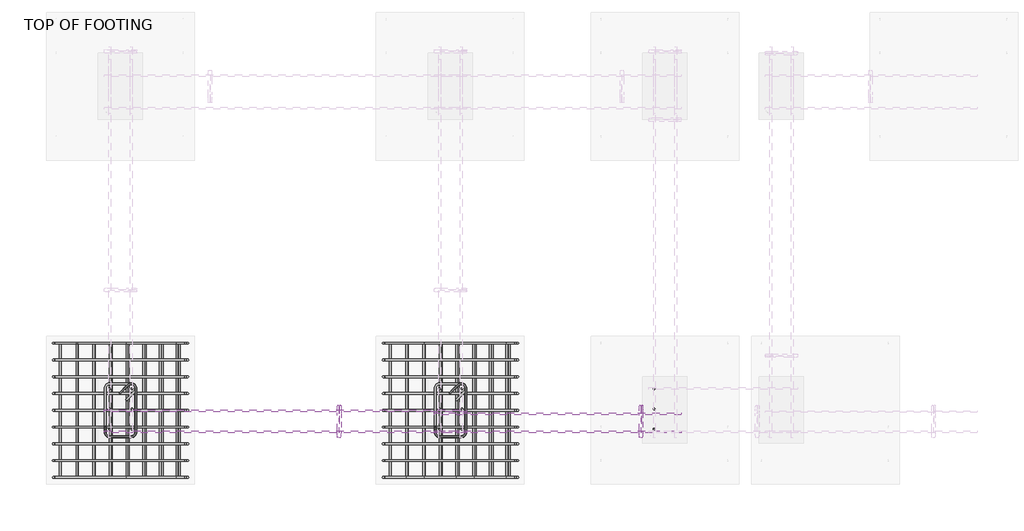
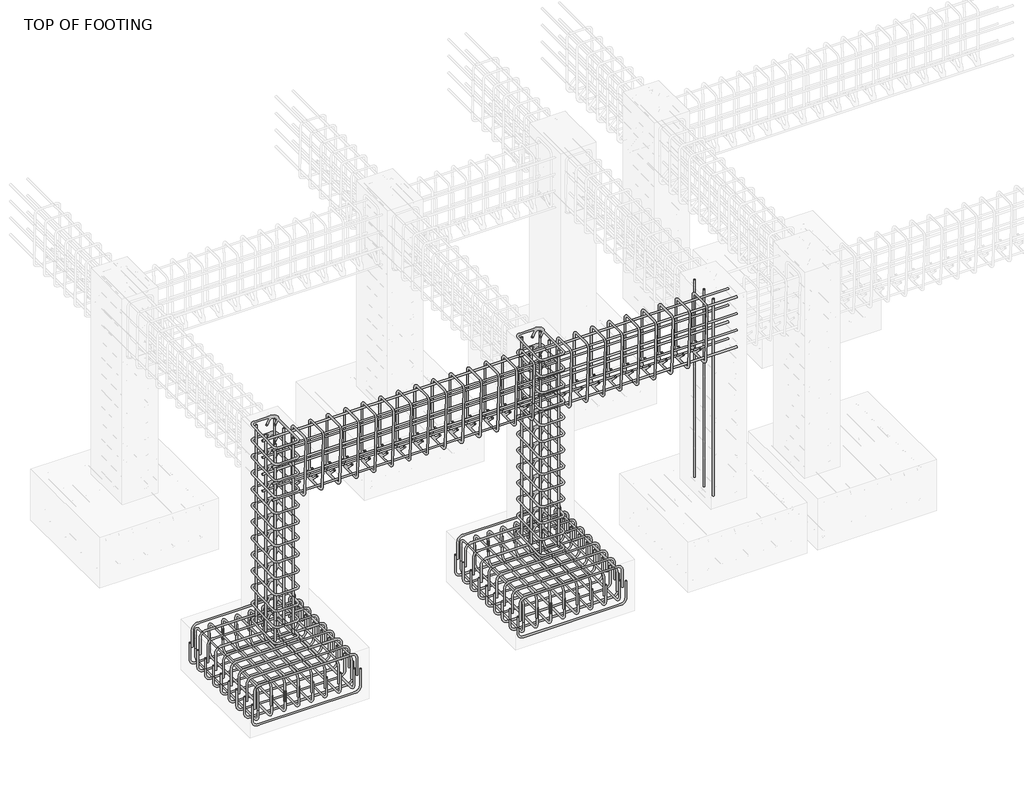
# One storey, part 2 of 19: 21 reinforcing bars.
"""IFC4 building model written with IfcOpenShell, lengths in millimetres."""

from ifc_helpers import new_model, si_unit, point, frame, origin, place, context, project, spatial, polyline, circle_curve, trimmed, segment, composite_curve, source, transform, mapped, element, save
from ifc_brep_helpers import swept_disk

model = new_model("IFC4")

# Units and contexts
model_context = context("Model", 3, world=origin())
ifc_project = project(units=[si_unit("LENGTHUNIT", "METRE", prefix="MILLI")], contexts=[model_context])

# Site, building, storey
site = spatial("IfcSite", under=ifc_project)
building = spatial("IfcBuilding", under=site)
storey = spatial("IfcBuildingStorey", under=building, Name="TOP OF FOOTING", Elevation=-1828.8)

# Reinforcing bars
placement = place(None, origin())
reinforcing_bar_shape = source(origin(), model_context, "Body", "SolidModel", [
    swept_disk(composite_curve([segment(polyline([(-5184.0266954, -464.2751006, -2026.8103972), (-5184.0266954, -464.2751006, -2174.1103972)]), True, "CONTINUOUS"), segment(trimmed(circle_curve(frame((-5230.3766954, -464.2751006, -2174.1103972), z_axis=(0.0, 1.0, 0.0), x_axis=(46.350000000000364, 0.0, 0.0)), 46.35), [point((-5184.0266954, -464.2751006, -2174.1103972))], [point((-5230.3766954, -464.2751006, -2220.4603972))], True, "CARTESIAN"), True, "CONTINUOUS"), segment(polyline([(-5230.3766954, -464.2751006, -2220.4603972), (-6044.9766954, -464.2751006, -2220.4603972)]), True, "CONTINUOUS"), segment(trimmed(circle_curve(frame((-6044.9766954, -464.2751006, -2174.1103972), z_axis=(0.0, 1.0, 0.0), x_axis=(0.0, 0.0, -46.34999999999991)), 46.35), [point((-6044.9766954, -464.2751006, -2220.4603972))], [point((-6091.3266954, -464.2751006, -2174.1103972))], True, "CARTESIAN"), True, "CONTINUOUS"), segment(polyline([(-6091.3266954, -464.2751006, -2174.1103972), (-6091.3266954, -464.2751006, -2026.8103972)]), True, "CONTINUOUS")], self_intersect=False), 6.35),
])
element("IfcReinforcingBar", 1, at=placement, inside=storey, context=model_context, shape_type="MappedRepresentation", body=[
    mapped(reinforcing_bar_shape, transform((0.0, 0.0, 0.0), x_axis=(1.0, 0.0, 0.0), y_axis=(0.0, 1.0, 0.0), z_axis=(0.0, 0.0, 1.0))),
    mapped(reinforcing_bar_shape, transform((0.0, -113.4125, 0.0), x_axis=(1.0, 0.0, 0.0), y_axis=(0.0, 1.0, 0.0), z_axis=(0.0, 0.0, 1.0))),
    mapped(reinforcing_bar_shape, transform((0.0, -226.825, 0.0), x_axis=(1.0, 0.0, 0.0), y_axis=(0.0, 1.0, 0.0), z_axis=(0.0, 0.0, 1.0))),
    mapped(reinforcing_bar_shape, transform((0.0, -340.2375, 0.0), x_axis=(1.0, 0.0, 0.0), y_axis=(0.0, 1.0, 0.0), z_axis=(0.0, 0.0, 1.0))),
    mapped(reinforcing_bar_shape, transform((0.0, -453.65, 0.0), x_axis=(1.0, 0.0, 0.0), y_axis=(0.0, 1.0, 0.0), z_axis=(0.0, 0.0, 1.0))),
    mapped(reinforcing_bar_shape, transform((0.0, -567.0625, 0.0), x_axis=(1.0, 0.0, 0.0), y_axis=(0.0, 1.0, 0.0), z_axis=(0.0, 0.0, 1.0))),
    mapped(reinforcing_bar_shape, transform((0.0, -680.475, 0.0), x_axis=(1.0, 0.0, 0.0), y_axis=(0.0, 1.0, 0.0), z_axis=(0.0, 0.0, 1.0))),
    mapped(reinforcing_bar_shape, transform((0.0, -793.8875, 0.0), x_axis=(1.0, 0.0, 0.0), y_axis=(0.0, 1.0, 0.0), z_axis=(0.0, 0.0, 1.0))),
    mapped(reinforcing_bar_shape, transform((0.0, -907.3, 0.0), x_axis=(1.0, 0.0, 0.0), y_axis=(0.0, 1.0, 0.0), z_axis=(0.0, 0.0, 1.0))),
])
reinforcing_bar_2_shape = source(origin(), model_context, "Body", "SolidModel", [
    swept_disk(composite_curve([segment(polyline([(-6071.7887242, -464.2751006, -2068.8), (-6071.7887242, -464.2751006, -1921.5)]), True, "CONTINUOUS"), segment(trimmed(circle_curve(frame((-6025.4387242, -464.2751006, -1921.5), z_axis=(0.0, 1.0, 0.0), x_axis=(-46.349999999999454, 0.0, 0.0)), 46.35), [point((-6071.7887242, -464.2751006, -1921.5))], [point((-6025.4387242, -464.2751006, -1875.15))], True, "CARTESIAN"), True, "CONTINUOUS"), segment(polyline([(-6025.4387242, -464.2751006, -1875.15), (-5260.3062054, -464.2751006, -1875.15)]), True, "CONTINUOUS"), segment(trimmed(circle_curve(frame((-5260.3062054, -464.2751006, -1921.5), z_axis=(0.0, 1.0, 0.0), x_axis=(0.0, 0.0, 46.34999999999991)), 46.35), [point((-5260.3062054, -464.2751006, -1875.15))], [point((-5213.9562054, -464.2751006, -1921.5))], True, "CARTESIAN"), True, "CONTINUOUS"), segment(polyline([(-5213.9562054, -464.2751006, -1921.5), (-5213.9562054, -464.2751006, -2068.8)]), True, "CONTINUOUS")], self_intersect=False), 6.35),
])
element("IfcReinforcingBar", 2, at=placement, inside=storey, context=model_context, shape_type="MappedRepresentation", body=[
    mapped(reinforcing_bar_2_shape, transform((0.0, 0.0, 0.0), x_axis=(1.0, 0.0, 0.0), y_axis=(0.0, 1.0, 0.0), z_axis=(0.0, 0.0, 1.0))),
    mapped(reinforcing_bar_2_shape, transform((0.0, -113.4125, 0.0), x_axis=(1.0, 0.0, 0.0), y_axis=(0.0, 1.0, 0.0), z_axis=(0.0, 0.0, 1.0))),
    mapped(reinforcing_bar_2_shape, transform((0.0, -226.825, 0.0), x_axis=(1.0, 0.0, 0.0), y_axis=(0.0, 1.0, 0.0), z_axis=(0.0, 0.0, 1.0))),
    mapped(reinforcing_bar_2_shape, transform((0.0, -340.2375, 0.0), x_axis=(1.0, 0.0, 0.0), y_axis=(0.0, 1.0, 0.0), z_axis=(0.0, 0.0, 1.0))),
    mapped(reinforcing_bar_2_shape, transform((0.0, -453.65, 0.0), x_axis=(1.0, 0.0, 0.0), y_axis=(0.0, 1.0, 0.0), z_axis=(0.0, 0.0, 1.0))),
    mapped(reinforcing_bar_2_shape, transform((0.0, -567.0625, 0.0), x_axis=(1.0, 0.0, 0.0), y_axis=(0.0, 1.0, 0.0), z_axis=(0.0, 0.0, 1.0))),
    mapped(reinforcing_bar_2_shape, transform((0.0, -680.475, 0.0), x_axis=(1.0, 0.0, 0.0), y_axis=(0.0, 1.0, 0.0), z_axis=(0.0, 0.0, 1.0))),
    mapped(reinforcing_bar_2_shape, transform((0.0, -793.8875, 0.0), x_axis=(1.0, 0.0, 0.0), y_axis=(0.0, 1.0, 0.0), z_axis=(0.0, 0.0, 1.0))),
    mapped(reinforcing_bar_2_shape, transform((0.0, -907.3, 0.0), x_axis=(1.0, 0.0, 0.0), y_axis=(0.0, 1.0, 0.0), z_axis=(0.0, 0.0, 1.0))),
])
reinforcing_bar_3_shape = source(origin(), model_context, "Body", "SolidModel", [
    swept_disk(composite_curve([segment(polyline([(-5256.531502, -464.2751006, -2090.0818702), (-5256.531502, -464.2751006, -1942.7818702)]), True, "CONTINUOUS"), segment(trimmed(circle_curve(frame((-5256.531502, -510.6251006, -1942.7818702), z_axis=(1.0, 0.0, 0.0), x_axis=(0.0, 46.35000000000002, 0.0)), 46.35), [point((-5256.531502, -464.2751006, -1942.7818702))], [point((-5256.531502, -510.6251006, -1896.4318702))], True, "CARTESIAN"), True, "CONTINUOUS"), segment(polyline([(-5256.531502, -510.6251006, -1896.4318702), (-5256.531502, -1325.2251006, -1896.4318702)]), True, "CONTINUOUS"), segment(trimmed(circle_curve(frame((-5256.531502, -1325.2251006, -1942.7818702), z_axis=(1.0, 0.0, 0.0), x_axis=(0.0, 0.0, 46.34999999999991)), 46.35), [point((-5256.531502, -1325.2251006, -1896.4318702))], [point((-5256.531502, -1371.5751006, -1942.7818702))], True, "CARTESIAN"), True, "CONTINUOUS"), segment(polyline([(-5256.531502, -1371.5751006, -1942.7818702), (-5256.531502, -1371.5751006, -2090.0818702)]), True, "CONTINUOUS")], self_intersect=False), 6.35),
])
element("IfcReinforcingBar", 3, at=placement, inside=storey, context=model_context, shape_type="MappedRepresentation", body=[
    mapped(reinforcing_bar_3_shape, transform((0.0, 0.0, 0.0), x_axis=(1.0, 0.0, 0.0), y_axis=(0.0, 1.0, 0.0), z_axis=(0.0, 0.0, 1.0))),
    mapped(reinforcing_bar_3_shape, transform((-112.5756498, 0.0, 0.0), x_axis=(1.0, 0.0, 0.0), y_axis=(0.0, 1.0, 0.0), z_axis=(0.0, 0.0, 1.0))),
    mapped(reinforcing_bar_3_shape, transform((-225.1512997, 0.0, 0.0), x_axis=(1.0, 0.0, 0.0), y_axis=(0.0, 1.0, 0.0), z_axis=(0.0, 0.0, 1.0))),
    mapped(reinforcing_bar_3_shape, transform((-337.7269495, 0.0, 0.0), x_axis=(1.0, 0.0, 0.0), y_axis=(0.0, 1.0, 0.0), z_axis=(0.0, 0.0, 1.0))),
    mapped(reinforcing_bar_3_shape, transform((-450.3025994, 0.0, 0.0), x_axis=(1.0, 0.0, 0.0), y_axis=(0.0, 1.0, 0.0), z_axis=(0.0, 0.0, 1.0))),
    mapped(reinforcing_bar_3_shape, transform((-562.8782492, 0.0, 0.0), x_axis=(1.0, 0.0, 0.0), y_axis=(0.0, 1.0, 0.0), z_axis=(0.0, 0.0, 1.0))),
    mapped(reinforcing_bar_3_shape, transform((-675.4538991, 0.0, 0.0), x_axis=(1.0, 0.0, 0.0), y_axis=(0.0, 1.0, 0.0), z_axis=(0.0, 0.0, 1.0))),
    mapped(reinforcing_bar_3_shape, transform((-788.0295489, 0.0, 0.0), x_axis=(1.0, 0.0, 0.0), y_axis=(0.0, 1.0, 0.0), z_axis=(0.0, 0.0, 1.0))),
])
reinforcing_bar_4_shape = source(origin(), model_context, "Body", "SolidModel", [
    swept_disk(composite_curve([segment(polyline([(-6044.5610509, -464.2751006, -2000.9061905), (-6044.5610509, -464.2751006, -2148.2061905)]), True, "CONTINUOUS"), segment(trimmed(circle_curve(frame((-6044.5610509, -510.6251006, -2148.2061905), z_axis=(-1.0, 0.0, 0.0), x_axis=(0.0, 46.35000000000002, 0.0)), 46.35), [point((-6044.5610509, -464.2751006, -2148.2061905))], [point((-6044.5610509, -510.6251006, -2194.5561905))], True, "CARTESIAN"), True, "CONTINUOUS"), segment(polyline([(-6044.5610509, -510.6251006, -2194.5561905), (-6044.5610509, -1325.2251006, -2194.5561905)]), True, "CONTINUOUS"), segment(trimmed(circle_curve(frame((-6044.5610509, -1325.2251006, -2148.2061905), z_axis=(-1.0, 0.0, 0.0), x_axis=(0.0, 0.0, -46.34999999999991)), 46.35), [point((-6044.5610509, -1325.2251006, -2194.5561905))], [point((-6044.5610509, -1371.5751006, -2148.2061905))], True, "CARTESIAN"), True, "CONTINUOUS"), segment(polyline([(-6044.5610509, -1371.5751006, -2148.2061905), (-6044.5610509, -1371.5751006, -2000.9061905)]), True, "CONTINUOUS")], self_intersect=False), 6.35),
])
element("IfcReinforcingBar", 4, at=placement, inside=storey, context=model_context, shape_type="MappedRepresentation", body=[
    mapped(reinforcing_bar_4_shape, transform((0.0, 0.0, 0.0), x_axis=(1.0, 0.0, 0.0), y_axis=(0.0, 1.0, 0.0), z_axis=(0.0, 0.0, 1.0))),
    mapped(reinforcing_bar_4_shape, transform((115.0727115, 0.0, 0.0), x_axis=(1.0, 0.0, 0.0), y_axis=(0.0, 1.0, 0.0), z_axis=(0.0, 0.0, 1.0))),
    mapped(reinforcing_bar_4_shape, transform((230.145423, 0.0, 0.0), x_axis=(1.0, 0.0, 0.0), y_axis=(0.0, 1.0, 0.0), z_axis=(0.0, 0.0, 1.0))),
    mapped(reinforcing_bar_4_shape, transform((345.2181344, 0.0, 0.0), x_axis=(1.0, 0.0, 0.0), y_axis=(0.0, 1.0, 0.0), z_axis=(0.0, 0.0, 1.0))),
    mapped(reinforcing_bar_4_shape, transform((460.2908459, 0.0, 0.0), x_axis=(1.0, 0.0, 0.0), y_axis=(0.0, 1.0, 0.0), z_axis=(0.0, 0.0, 1.0))),
    mapped(reinforcing_bar_4_shape, transform((575.3635574, 0.0, 0.0), x_axis=(1.0, 0.0, 0.0), y_axis=(0.0, 1.0, 0.0), z_axis=(0.0, 0.0, 1.0))),
    mapped(reinforcing_bar_4_shape, transform((690.4362689, 0.0, 0.0), x_axis=(1.0, 0.0, 0.0), y_axis=(0.0, 1.0, 0.0), z_axis=(0.0, 0.0, 1.0))),
    mapped(reinforcing_bar_4_shape, transform((805.5089804, 0.0, 0.0), x_axis=(1.0, 0.0, 0.0), y_axis=(0.0, 1.0, 0.0), z_axis=(0.0, 0.0, 1.0))),
])
reinforcing_bar_5_shape = source(origin(), model_context, "Body", "SolidModel", [
    swept_disk(composite_curve([segment(polyline([(-2954.6283472, -464.2751006, -2026.8103972), (-2954.6283472, -464.2751006, -2174.1103972)]), True, "CONTINUOUS"), segment(trimmed(circle_curve(frame((-3000.9783472, -464.2751006, -2174.1103972), z_axis=(0.0, 1.0, 0.0), x_axis=(46.34999999999991, 0.0, 0.0)), 46.35), [point((-2954.6283472, -464.2751006, -2174.1103972))], [point((-3000.9783472, -464.2751006, -2220.4603972))], True, "CARTESIAN"), True, "CONTINUOUS"), segment(polyline([(-3000.9783472, -464.2751006, -2220.4603972), (-3815.5783472, -464.2751006, -2220.4603972)]), True, "CONTINUOUS"), segment(trimmed(circle_curve(frame((-3815.5783472, -464.2751006, -2174.1103972), z_axis=(0.0, 1.0, 0.0), x_axis=(0.0, 0.0, -46.34999999999991)), 46.35), [point((-3815.5783472, -464.2751006, -2220.4603972))], [point((-3861.9283472, -464.2751006, -2174.1103972))], True, "CARTESIAN"), True, "CONTINUOUS"), segment(polyline([(-3861.9283472, -464.2751006, -2174.1103972), (-3861.9283472, -464.2751006, -2026.8103972)]), True, "CONTINUOUS")], self_intersect=False), 6.35),
])
element("IfcReinforcingBar", 5, at=placement, inside=storey, context=model_context, shape_type="MappedRepresentation", body=[
    mapped(reinforcing_bar_5_shape, transform((0.0, 0.0, 0.0), x_axis=(1.0, 0.0, 0.0), y_axis=(0.0, 1.0, 0.0), z_axis=(0.0, 0.0, 1.0))),
    mapped(reinforcing_bar_5_shape, transform((0.0, -113.4125, 0.0), x_axis=(1.0, 0.0, 0.0), y_axis=(0.0, 1.0, 0.0), z_axis=(0.0, 0.0, 1.0))),
    mapped(reinforcing_bar_5_shape, transform((0.0, -226.825, 0.0), x_axis=(1.0, 0.0, 0.0), y_axis=(0.0, 1.0, 0.0), z_axis=(0.0, 0.0, 1.0))),
    mapped(reinforcing_bar_5_shape, transform((0.0, -340.2375, 0.0), x_axis=(1.0, 0.0, 0.0), y_axis=(0.0, 1.0, 0.0), z_axis=(0.0, 0.0, 1.0))),
    mapped(reinforcing_bar_5_shape, transform((0.0, -453.65, 0.0), x_axis=(1.0, 0.0, 0.0), y_axis=(0.0, 1.0, 0.0), z_axis=(0.0, 0.0, 1.0))),
    mapped(reinforcing_bar_5_shape, transform((0.0, -567.0625, 0.0), x_axis=(1.0, 0.0, 0.0), y_axis=(0.0, 1.0, 0.0), z_axis=(0.0, 0.0, 1.0))),
    mapped(reinforcing_bar_5_shape, transform((0.0, -680.475, 0.0), x_axis=(1.0, 0.0, 0.0), y_axis=(0.0, 1.0, 0.0), z_axis=(0.0, 0.0, 1.0))),
    mapped(reinforcing_bar_5_shape, transform((0.0, -793.8875, 0.0), x_axis=(1.0, 0.0, 0.0), y_axis=(0.0, 1.0, 0.0), z_axis=(0.0, 0.0, 1.0))),
    mapped(reinforcing_bar_5_shape, transform((0.0, -907.3, 0.0), x_axis=(1.0, 0.0, 0.0), y_axis=(0.0, 1.0, 0.0), z_axis=(0.0, 0.0, 1.0))),
])
reinforcing_bar_6_shape = source(origin(), model_context, "Body", "SolidModel", [
    swept_disk(composite_curve([segment(polyline([(-3842.390376, -464.2751006, -2068.8), (-3842.390376, -464.2751006, -1921.5)]), True, "CONTINUOUS"), segment(trimmed(circle_curve(frame((-3796.040376, -464.2751006, -1921.5), z_axis=(0.0, 1.0, 0.0), x_axis=(-46.34999999999991, 0.0, 0.0)), 46.35), [point((-3842.390376, -464.2751006, -1921.5))], [point((-3796.040376, -464.2751006, -1875.15))], True, "CARTESIAN"), True, "CONTINUOUS"), segment(polyline([(-3796.040376, -464.2751006, -1875.15), (-3030.9078572, -464.2751006, -1875.15)]), True, "CONTINUOUS"), segment(trimmed(circle_curve(frame((-3030.9078572, -464.2751006, -1921.5), z_axis=(0.0, 1.0, 0.0), x_axis=(0.0, 0.0, 46.34999999999991)), 46.35), [point((-3030.9078572, -464.2751006, -1875.15))], [point((-2984.5578572, -464.2751006, -1921.5))], True, "CARTESIAN"), True, "CONTINUOUS"), segment(polyline([(-2984.5578572, -464.2751006, -1921.5), (-2984.5578572, -464.2751006, -2068.8)]), True, "CONTINUOUS")], self_intersect=False), 6.35),
])
element("IfcReinforcingBar", 6, at=placement, inside=storey, context=model_context, shape_type="MappedRepresentation", body=[
    mapped(reinforcing_bar_6_shape, transform((0.0, 0.0, 0.0), x_axis=(1.0, 0.0, 0.0), y_axis=(0.0, 1.0, 0.0), z_axis=(0.0, 0.0, 1.0))),
    mapped(reinforcing_bar_6_shape, transform((0.0, -113.4125, 0.0), x_axis=(1.0, 0.0, 0.0), y_axis=(0.0, 1.0, 0.0), z_axis=(0.0, 0.0, 1.0))),
    mapped(reinforcing_bar_6_shape, transform((0.0, -226.825, 0.0), x_axis=(1.0, 0.0, 0.0), y_axis=(0.0, 1.0, 0.0), z_axis=(0.0, 0.0, 1.0))),
    mapped(reinforcing_bar_6_shape, transform((0.0, -340.2375, 0.0), x_axis=(1.0, 0.0, 0.0), y_axis=(0.0, 1.0, 0.0), z_axis=(0.0, 0.0, 1.0))),
    mapped(reinforcing_bar_6_shape, transform((0.0, -453.65, 0.0), x_axis=(1.0, 0.0, 0.0), y_axis=(0.0, 1.0, 0.0), z_axis=(0.0, 0.0, 1.0))),
    mapped(reinforcing_bar_6_shape, transform((0.0, -567.0625, 0.0), x_axis=(1.0, 0.0, 0.0), y_axis=(0.0, 1.0, 0.0), z_axis=(0.0, 0.0, 1.0))),
    mapped(reinforcing_bar_6_shape, transform((0.0, -680.475, 0.0), x_axis=(1.0, 0.0, 0.0), y_axis=(0.0, 1.0, 0.0), z_axis=(0.0, 0.0, 1.0))),
    mapped(reinforcing_bar_6_shape, transform((0.0, -793.8875, 0.0), x_axis=(1.0, 0.0, 0.0), y_axis=(0.0, 1.0, 0.0), z_axis=(0.0, 0.0, 1.0))),
    mapped(reinforcing_bar_6_shape, transform((0.0, -907.3, 0.0), x_axis=(1.0, 0.0, 0.0), y_axis=(0.0, 1.0, 0.0), z_axis=(0.0, 0.0, 1.0))),
])
reinforcing_bar_7_shape = source(origin(), model_context, "Body", "SolidModel", [
    swept_disk(composite_curve([segment(polyline([(-3027.1331538, -464.2751006, -2090.0818702), (-3027.1331538, -464.2751006, -1942.7818702)]), True, "CONTINUOUS"), segment(trimmed(circle_curve(frame((-3027.1331538, -510.6251006, -1942.7818702), z_axis=(1.0, 0.0, 0.0), x_axis=(0.0, 46.35000000000002, 0.0)), 46.35), [point((-3027.1331538, -464.2751006, -1942.7818702))], [point((-3027.1331538, -510.6251006, -1896.4318702))], True, "CARTESIAN"), True, "CONTINUOUS"), segment(polyline([(-3027.1331538, -510.6251006, -1896.4318702), (-3027.1331538, -1325.2251006, -1896.4318702)]), True, "CONTINUOUS"), segment(trimmed(circle_curve(frame((-3027.1331538, -1325.2251006, -1942.7818702), z_axis=(1.0, 0.0, 0.0), x_axis=(0.0, 0.0, 46.34999999999991)), 46.35), [point((-3027.1331538, -1325.2251006, -1896.4318702))], [point((-3027.1331538, -1371.5751006, -1942.7818702))], True, "CARTESIAN"), True, "CONTINUOUS"), segment(polyline([(-3027.1331538, -1371.5751006, -1942.7818702), (-3027.1331538, -1371.5751006, -2090.0818702)]), True, "CONTINUOUS")], self_intersect=False), 6.35),
])
element("IfcReinforcingBar", 7, at=placement, inside=storey, context=model_context, shape_type="MappedRepresentation", body=[
    mapped(reinforcing_bar_7_shape, transform((0.0, 0.0, 0.0), x_axis=(1.0, 0.0, 0.0), y_axis=(0.0, 1.0, 0.0), z_axis=(0.0, 0.0, 1.0))),
    mapped(reinforcing_bar_7_shape, transform((-112.5756498, 0.0, 0.0), x_axis=(1.0, 0.0, 0.0), y_axis=(0.0, 1.0, 0.0), z_axis=(0.0, 0.0, 1.0))),
    mapped(reinforcing_bar_7_shape, transform((-225.1512997, 0.0, 0.0), x_axis=(1.0, 0.0, 0.0), y_axis=(0.0, 1.0, 0.0), z_axis=(0.0, 0.0, 1.0))),
    mapped(reinforcing_bar_7_shape, transform((-337.7269495, 0.0, 0.0), x_axis=(1.0, 0.0, 0.0), y_axis=(0.0, 1.0, 0.0), z_axis=(0.0, 0.0, 1.0))),
    mapped(reinforcing_bar_7_shape, transform((-450.3025994, 0.0, 0.0), x_axis=(1.0, 0.0, 0.0), y_axis=(0.0, 1.0, 0.0), z_axis=(0.0, 0.0, 1.0))),
    mapped(reinforcing_bar_7_shape, transform((-562.8782492, 0.0, 0.0), x_axis=(1.0, 0.0, 0.0), y_axis=(0.0, 1.0, 0.0), z_axis=(0.0, 0.0, 1.0))),
    mapped(reinforcing_bar_7_shape, transform((-675.4538991, 0.0, 0.0), x_axis=(1.0, 0.0, 0.0), y_axis=(0.0, 1.0, 0.0), z_axis=(0.0, 0.0, 1.0))),
    mapped(reinforcing_bar_7_shape, transform((-788.0295489, 0.0, 0.0), x_axis=(1.0, 0.0, 0.0), y_axis=(0.0, 1.0, 0.0), z_axis=(0.0, 0.0, 1.0))),
])
reinforcing_bar_8_shape = source(origin(), model_context, "Body", "SolidModel", [
    swept_disk(composite_curve([segment(polyline([(-3815.1627027, -464.2751006, -2000.9061905), (-3815.1627027, -464.2751006, -2148.2061905)]), True, "CONTINUOUS"), segment(trimmed(circle_curve(frame((-3815.1627027, -510.6251006, -2148.2061905), z_axis=(-1.0, 0.0, 0.0), x_axis=(0.0, 46.35000000000002, 0.0)), 46.35), [point((-3815.1627027, -464.2751006, -2148.2061905))], [point((-3815.1627027, -510.6251006, -2194.5561905))], True, "CARTESIAN"), True, "CONTINUOUS"), segment(polyline([(-3815.1627027, -510.6251006, -2194.5561905), (-3815.1627027, -1325.2251006, -2194.5561905)]), True, "CONTINUOUS"), segment(trimmed(circle_curve(frame((-3815.1627027, -1325.2251006, -2148.2061905), z_axis=(-1.0, 0.0, 0.0), x_axis=(0.0, 0.0, -46.34999999999991)), 46.35), [point((-3815.1627027, -1325.2251006, -2194.5561905))], [point((-3815.1627027, -1371.5751006, -2148.2061905))], True, "CARTESIAN"), True, "CONTINUOUS"), segment(polyline([(-3815.1627027, -1371.5751006, -2148.2061905), (-3815.1627027, -1371.5751006, -2000.9061905)]), True, "CONTINUOUS")], self_intersect=False), 6.35),
])
element("IfcReinforcingBar", 8, at=placement, inside=storey, context=model_context, shape_type="MappedRepresentation", body=[
    mapped(reinforcing_bar_8_shape, transform((0.0, 0.0, 0.0), x_axis=(1.0, 0.0, 0.0), y_axis=(0.0, 1.0, 0.0), z_axis=(0.0, 0.0, 1.0))),
    mapped(reinforcing_bar_8_shape, transform((115.0727115, 0.0, 0.0), x_axis=(1.0, 0.0, 0.0), y_axis=(0.0, 1.0, 0.0), z_axis=(0.0, 0.0, 1.0))),
    mapped(reinforcing_bar_8_shape, transform((230.145423, 0.0, 0.0), x_axis=(1.0, 0.0, 0.0), y_axis=(0.0, 1.0, 0.0), z_axis=(0.0, 0.0, 1.0))),
    mapped(reinforcing_bar_8_shape, transform((345.2181344, 0.0, 0.0), x_axis=(1.0, 0.0, 0.0), y_axis=(0.0, 1.0, 0.0), z_axis=(0.0, 0.0, 1.0))),
    mapped(reinforcing_bar_8_shape, transform((460.2908459, 0.0, 0.0), x_axis=(1.0, 0.0, 0.0), y_axis=(0.0, 1.0, 0.0), z_axis=(0.0, 0.0, 1.0))),
    mapped(reinforcing_bar_8_shape, transform((575.3635574, 0.0, 0.0), x_axis=(1.0, 0.0, 0.0), y_axis=(0.0, 1.0, 0.0), z_axis=(0.0, 0.0, 1.0))),
    mapped(reinforcing_bar_8_shape, transform((690.4362689, 0.0, 0.0), x_axis=(1.0, 0.0, 0.0), y_axis=(0.0, 1.0, 0.0), z_axis=(0.0, 0.0, 1.0))),
    mapped(reinforcing_bar_8_shape, transform((805.5089804, 0.0, 0.0), x_axis=(1.0, 0.0, 0.0), y_axis=(0.0, 1.0, 0.0), z_axis=(0.0, 0.0, 1.0))),
])
reinforcing_bar_9_shape = source(origin(), model_context, "Body", "SolidModel", [
    swept_disk(composite_curve([segment(polyline([(-5643.2880559, -804.200866, -46.35), (-5587.544493, -748.457303, -46.35)]), True, "CONTINUOUS"), segment(trimmed(circle_curve(frame((-5565.3766954, -770.6251006, -46.35), z_axis=(0.0, 0.0, -1.0), x_axis=(-22.167797600000085, 22.16779759999997, 0.0)), 31.35), [point((-5587.544493, -748.457303, -46.35))], [point((-5534.0266954, -770.6251006, -46.35))], True, "CARTESIAN"), True, "CONTINUOUS"), segment(polyline([(-5534.0266954, -770.6251006, -46.35), (-5534.0266954, -1065.2251006, -46.35)]), True, "CONTINUOUS"), segment(trimmed(circle_curve(frame((-5565.3766954, -1065.2251006, -46.35), z_axis=(0.0, 0.0, -1.0), x_axis=(31.350000000000364, 0.0, 0.0)), 31.35), [point((-5534.0266954, -1065.2251006, -46.35))], [point((-5565.3766954, -1096.5751006, -46.35))], True, "CARTESIAN"), True, "CONTINUOUS"), segment(polyline([(-5565.3766954, -1096.5751006, -46.35), (-5709.9766954, -1096.5751006, -46.35)]), True, "CONTINUOUS"), segment(trimmed(circle_curve(frame((-5709.9766954, -1065.2448857, -45.2363875), z_axis=(0.0, 0.035521928334481916, -0.9993688971583016), x_axis=(0.0, -31.3302149000001, -1.1136125000000021)), 31.35), [point((-5709.9766954, -1096.5751006, -46.35))], [point((-5741.3266954, -1065.2448857, -45.2363875))], True, "CARTESIAN"), True, "CONTINUOUS"), segment(polyline([(-5741.3266954, -1065.2448857, -45.2363875), (-5741.3266954, -770.6053156, -34.7636125)]), True, "CONTINUOUS"), segment(trimmed(circle_curve(frame((-5709.9766954, -770.6053156, -34.7636125), z_axis=(0.0, 0.035521928334481916, -0.9993688971583016), x_axis=(-31.350000000000364, 0.0, 0.0)), 31.35), [point((-5741.3266954, -770.6053156, -34.7636125))], [point((-5709.9766954, -739.2751006, -33.65))], True, "CARTESIAN"), True, "CONTINUOUS"), segment(polyline([(-5709.9766954, -739.2751006, -33.65), (-5565.3766954, -739.2751006, -33.65)]), True, "CONTINUOUS"), segment(trimmed(circle_curve(frame((-5565.3766954, -770.6251006, -33.65), z_axis=(0.0, 0.0, -1.0), x_axis=(0.0, 31.350000000000023, 0.0)), 31.35), [point((-5565.3766954, -739.2751006, -33.65))], [point((-5543.2088978, -792.7928982, -33.65))], True, "CARTESIAN"), True, "CONTINUOUS"), segment(polyline([(-5543.2088978, -792.7928982, -33.65), (-5598.9524607, -848.5364612, -33.65)]), True, "CONTINUOUS")], self_intersect=False), 6.35),
])
element("IfcReinforcingBar", 9, at=placement, inside=storey, context=model_context, shape_type="MappedRepresentation", body=[
    mapped(reinforcing_bar_9_shape, transform((0.0, 0.0, 0.0), x_axis=(1.0, 0.0, 0.0), y_axis=(0.0, 1.0, 0.0), z_axis=(0.0, 0.0, 1.0))),
    mapped(reinforcing_bar_9_shape, transform((0.0, 0.0, -144.675), x_axis=(1.0, 0.0, 0.0), y_axis=(0.0, 1.0, 0.0), z_axis=(0.0, 0.0, 1.0))),
    mapped(reinforcing_bar_9_shape, transform((0.0, 0.0, -289.35), x_axis=(1.0, 0.0, 0.0), y_axis=(0.0, 1.0, 0.0), z_axis=(0.0, 0.0, 1.0))),
    mapped(reinforcing_bar_9_shape, transform((0.0, 0.0, -434.025), x_axis=(1.0, 0.0, 0.0), y_axis=(0.0, 1.0, 0.0), z_axis=(0.0, 0.0, 1.0))),
    mapped(reinforcing_bar_9_shape, transform((0.0, 0.0, -578.7), x_axis=(1.0, 0.0, 0.0), y_axis=(0.0, 1.0, 0.0), z_axis=(0.0, 0.0, 1.0))),
    mapped(reinforcing_bar_9_shape, transform((0.0, 0.0, -723.375), x_axis=(1.0, 0.0, 0.0), y_axis=(0.0, 1.0, 0.0), z_axis=(0.0, 0.0, 1.0))),
    mapped(reinforcing_bar_9_shape, transform((0.0, 0.0, -868.05), x_axis=(1.0, 0.0, 0.0), y_axis=(0.0, 1.0, 0.0), z_axis=(0.0, 0.0, 1.0))),
    mapped(reinforcing_bar_9_shape, transform((0.0, 0.0, -1012.725), x_axis=(1.0, 0.0, 0.0), y_axis=(0.0, 1.0, 0.0), z_axis=(0.0, 0.0, 1.0))),
    mapped(reinforcing_bar_9_shape, transform((0.0, 0.0, -1157.4), x_axis=(1.0, 0.0, 0.0), y_axis=(0.0, 1.0, 0.0), z_axis=(0.0, 0.0, 1.0))),
    mapped(reinforcing_bar_9_shape, transform((0.0, 0.0, -1302.075), x_axis=(1.0, 0.0, 0.0), y_axis=(0.0, 1.0, 0.0), z_axis=(0.0, 0.0, 1.0))),
    mapped(reinforcing_bar_9_shape, transform((0.0, 0.0, -1446.75), x_axis=(1.0, 0.0, 0.0), y_axis=(0.0, 1.0, 0.0), z_axis=(0.0, 0.0, 1.0))),
    mapped(reinforcing_bar_9_shape, transform((0.0, 0.0, -1591.425), x_axis=(1.0, 0.0, 0.0), y_axis=(0.0, 1.0, 0.0), z_axis=(0.0, 0.0, 1.0))),
    mapped(reinforcing_bar_9_shape, transform((0.0, 0.0, -1736.1), x_axis=(1.0, 0.0, 0.0), y_axis=(0.0, 1.0, 0.0), z_axis=(0.0, 0.0, 1.0))),
])
reinforcing_bar_10_shape = source(origin(), model_context, "Body", "SolidModel", [
    swept_disk(composite_curve([segment(polyline([(-5560.3766954, -772.4299352, -40.0), (-5560.3766954, -772.4299352, -1788.8)]), True, "CONTINUOUS")], self_intersect=False), 6.35),
])
element("IfcReinforcingBar", 10, at=placement, inside=storey, context=model_context, shape_type="MappedRepresentation", body=[
    mapped(reinforcing_bar_10_shape, transform((0.0, 0.0, 0.0), x_axis=(1.0, 0.0, 0.0), y_axis=(0.0, 1.0, 0.0), z_axis=(0.0, 0.0, 1.0))),
    mapped(reinforcing_bar_10_shape, transform((0.0, -136.8171118, 0.0), x_axis=(1.0, 0.0, 0.0), y_axis=(0.0, 1.0, 0.0), z_axis=(0.0, 0.0, 1.0))),
    mapped(reinforcing_bar_10_shape, transform((0.0, -273.6342236, 0.0), x_axis=(1.0, 0.0, 0.0), y_axis=(0.0, 1.0, 0.0), z_axis=(0.0, 0.0, 1.0))),
])
reinforcing_bar_11_shape = source(origin(), model_context, "Body", "SolidModel", [
    swept_disk(composite_curve([segment(polyline([(-5712.4766954, -772.4299352, -40.0), (-5712.4766954, -772.4299352, -1788.8)]), True, "CONTINUOUS")], self_intersect=False), 6.35),
])
element("IfcReinforcingBar", 11, at=placement, inside=storey, context=model_context, shape_type="MappedRepresentation", body=[
    mapped(reinforcing_bar_11_shape, transform((0.0, 0.0, 0.0), x_axis=(1.0, 0.0, 0.0), y_axis=(0.0, 1.0, 0.0), z_axis=(0.0, 0.0, 1.0))),
    mapped(reinforcing_bar_11_shape, transform((0.0, -136.8171118, 0.0), x_axis=(1.0, 0.0, 0.0), y_axis=(0.0, 1.0, 0.0), z_axis=(0.0, 0.0, 1.0))),
    mapped(reinforcing_bar_11_shape, transform((0.0, -273.6342236, 0.0), x_axis=(1.0, 0.0, 0.0), y_axis=(0.0, 1.0, 0.0), z_axis=(0.0, 0.0, 1.0))),
])
reinforcing_bar_12_shape = source(origin(), model_context, "Body", "SolidModel", [
    swept_disk(composite_curve([segment(polyline([(-3413.8897077, -804.200866, -46.35), (-3358.1461448, -748.457303, -46.35)]), True, "CONTINUOUS"), segment(trimmed(circle_curve(frame((-3335.9783472, -770.6251006, -46.35), z_axis=(0.0, 0.0, -1.0), x_axis=(-22.167797600000085, 22.16779759999997, 0.0)), 31.35), [point((-3358.1461448, -748.457303, -46.35))], [point((-3304.6283472, -770.6251006, -46.35))], True, "CARTESIAN"), True, "CONTINUOUS"), segment(polyline([(-3304.6283472, -770.6251006, -46.35), (-3304.6283472, -1065.2251006, -46.35)]), True, "CONTINUOUS"), segment(trimmed(circle_curve(frame((-3335.9783472, -1065.2251006, -46.35), z_axis=(0.0, 0.0, -1.0), x_axis=(31.34999999999991, 0.0, 0.0)), 31.35), [point((-3304.6283472, -1065.2251006, -46.35))], [point((-3335.9783472, -1096.5751006, -46.35))], True, "CARTESIAN"), True, "CONTINUOUS"), segment(polyline([(-3335.9783472, -1096.5751006, -46.35), (-3480.5783472, -1096.5751006, -46.35)]), True, "CONTINUOUS"), segment(trimmed(circle_curve(frame((-3480.5783472, -1065.2448857, -45.2363875), z_axis=(0.0, 0.035521928334481916, -0.9993688971583016), x_axis=(0.0, -31.3302149000001, -1.1136125000000021)), 31.35), [point((-3480.5783472, -1096.5751006, -46.35))], [point((-3511.9283472, -1065.2448857, -45.2363875))], True, "CARTESIAN"), True, "CONTINUOUS"), segment(polyline([(-3511.9283472, -1065.2448857, -45.2363875), (-3511.9283472, -770.6053156, -34.7636125)]), True, "CONTINUOUS"), segment(trimmed(circle_curve(frame((-3480.5783472, -770.6053156, -34.7636125), z_axis=(0.0, 0.035521928334481916, -0.9993688971583016), x_axis=(-31.350000000000364, 0.0, 0.0)), 31.35), [point((-3511.9283472, -770.6053156, -34.7636125))], [point((-3480.5783472, -739.2751006, -33.65))], True, "CARTESIAN"), True, "CONTINUOUS"), segment(polyline([(-3480.5783472, -739.2751006, -33.65), (-3335.9783472, -739.2751006, -33.65)]), True, "CONTINUOUS"), segment(trimmed(circle_curve(frame((-3335.9783472, -770.6251006, -33.65), z_axis=(0.0, 0.0, -1.0), x_axis=(0.0, 31.350000000000023, 0.0)), 31.35), [point((-3335.9783472, -739.2751006, -33.65))], [point((-3313.8105496, -792.7928982, -33.65))], True, "CARTESIAN"), True, "CONTINUOUS"), segment(polyline([(-3313.8105496, -792.7928982, -33.65), (-3369.5541126, -848.5364612, -33.65)]), True, "CONTINUOUS")], self_intersect=False), 6.35),
])
element("IfcReinforcingBar", 12, at=placement, inside=storey, context=model_context, shape_type="MappedRepresentation", body=[
    mapped(reinforcing_bar_12_shape, transform((0.0, 0.0, 0.0), x_axis=(1.0, 0.0, 0.0), y_axis=(0.0, 1.0, 0.0), z_axis=(0.0, 0.0, 1.0))),
    mapped(reinforcing_bar_12_shape, transform((0.0, 0.0, -144.675), x_axis=(1.0, 0.0, 0.0), y_axis=(0.0, 1.0, 0.0), z_axis=(0.0, 0.0, 1.0))),
    mapped(reinforcing_bar_12_shape, transform((0.0, 0.0, -289.35), x_axis=(1.0, 0.0, 0.0), y_axis=(0.0, 1.0, 0.0), z_axis=(0.0, 0.0, 1.0))),
    mapped(reinforcing_bar_12_shape, transform((0.0, 0.0, -434.025), x_axis=(1.0, 0.0, 0.0), y_axis=(0.0, 1.0, 0.0), z_axis=(0.0, 0.0, 1.0))),
    mapped(reinforcing_bar_12_shape, transform((0.0, 0.0, -578.7), x_axis=(1.0, 0.0, 0.0), y_axis=(0.0, 1.0, 0.0), z_axis=(0.0, 0.0, 1.0))),
    mapped(reinforcing_bar_12_shape, transform((0.0, 0.0, -723.375), x_axis=(1.0, 0.0, 0.0), y_axis=(0.0, 1.0, 0.0), z_axis=(0.0, 0.0, 1.0))),
    mapped(reinforcing_bar_12_shape, transform((0.0, 0.0, -868.05), x_axis=(1.0, 0.0, 0.0), y_axis=(0.0, 1.0, 0.0), z_axis=(0.0, 0.0, 1.0))),
    mapped(reinforcing_bar_12_shape, transform((0.0, 0.0, -1012.725), x_axis=(1.0, 0.0, 0.0), y_axis=(0.0, 1.0, 0.0), z_axis=(0.0, 0.0, 1.0))),
    mapped(reinforcing_bar_12_shape, transform((0.0, 0.0, -1157.4), x_axis=(1.0, 0.0, 0.0), y_axis=(0.0, 1.0, 0.0), z_axis=(0.0, 0.0, 1.0))),
    mapped(reinforcing_bar_12_shape, transform((0.0, 0.0, -1302.075), x_axis=(1.0, 0.0, 0.0), y_axis=(0.0, 1.0, 0.0), z_axis=(0.0, 0.0, 1.0))),
    mapped(reinforcing_bar_12_shape, transform((0.0, 0.0, -1446.75), x_axis=(1.0, 0.0, 0.0), y_axis=(0.0, 1.0, 0.0), z_axis=(0.0, 0.0, 1.0))),
    mapped(reinforcing_bar_12_shape, transform((0.0, 0.0, -1591.425), x_axis=(1.0, 0.0, 0.0), y_axis=(0.0, 1.0, 0.0), z_axis=(0.0, 0.0, 1.0))),
    mapped(reinforcing_bar_12_shape, transform((0.0, 0.0, -1736.1), x_axis=(1.0, 0.0, 0.0), y_axis=(0.0, 1.0, 0.0), z_axis=(0.0, 0.0, 1.0))),
])
reinforcing_bar_13_shape = source(origin(), model_context, "Body", "SolidModel", [
    swept_disk(composite_curve([segment(polyline([(-3330.9783472, -772.4299352, -40.0), (-3330.9783472, -772.4299352, -1788.8)]), True, "CONTINUOUS")], self_intersect=False), 6.35),
])
element("IfcReinforcingBar", 13, at=placement, inside=storey, context=model_context, shape_type="MappedRepresentation", body=[
    mapped(reinforcing_bar_13_shape, transform((0.0, 0.0, 0.0), x_axis=(1.0, 0.0, 0.0), y_axis=(0.0, 1.0, 0.0), z_axis=(0.0, 0.0, 1.0))),
    mapped(reinforcing_bar_13_shape, transform((0.0, -136.8171118, 0.0), x_axis=(1.0, 0.0, 0.0), y_axis=(0.0, 1.0, 0.0), z_axis=(0.0, 0.0, 1.0))),
    mapped(reinforcing_bar_13_shape, transform((0.0, -273.6342236, 0.0), x_axis=(1.0, 0.0, 0.0), y_axis=(0.0, 1.0, 0.0), z_axis=(0.0, 0.0, 1.0))),
])
reinforcing_bar_14_shape = source(origin(), model_context, "Body", "SolidModel", [
    swept_disk(composite_curve([segment(polyline([(-3483.0783472, -772.4299352, -40.0), (-3483.0783472, -772.4299352, -1788.8)]), True, "CONTINUOUS")], self_intersect=False), 6.35),
])
element("IfcReinforcingBar", 14, at=placement, inside=storey, context=model_context, shape_type="MappedRepresentation", body=[
    mapped(reinforcing_bar_14_shape, transform((0.0, 0.0, 0.0), x_axis=(1.0, 0.0, 0.0), y_axis=(0.0, 1.0, 0.0), z_axis=(0.0, 0.0, 1.0))),
    mapped(reinforcing_bar_14_shape, transform((0.0, -136.8171118, 0.0), x_axis=(1.0, 0.0, 0.0), y_axis=(0.0, 1.0, 0.0), z_axis=(0.0, 0.0, 1.0))),
    mapped(reinforcing_bar_14_shape, transform((0.0, -273.6342236, 0.0), x_axis=(1.0, 0.0, 0.0), y_axis=(0.0, 1.0, 0.0), z_axis=(0.0, 0.0, 1.0))),
])
reinforcing_bar_15_shape = source(origin(), model_context, "Body", "SolidModel", [
    swept_disk(composite_curve([segment(polyline([(-2032.4766954, -772.4299352, -40.0), (-2032.4766954, -772.4299352, -1788.8)]), True, "CONTINUOUS")], self_intersect=False), 6.35),
])
element("IfcReinforcingBar", 15, at=placement, inside=storey, context=model_context, shape_type="MappedRepresentation", body=[
    mapped(reinforcing_bar_15_shape, transform((0.0, 0.0, 0.0), x_axis=(1.0, 0.0, 0.0), y_axis=(0.0, 1.0, 0.0), z_axis=(0.0, 0.0, 1.0))),
    mapped(reinforcing_bar_15_shape, transform((0.0, -136.8171118, 0.0), x_axis=(1.0, 0.0, 0.0), y_axis=(0.0, 1.0, 0.0), z_axis=(0.0, 0.0, 1.0))),
    mapped(reinforcing_bar_15_shape, transform((0.0, -273.6342236, 0.0), x_axis=(1.0, 0.0, 0.0), y_axis=(0.0, 1.0, 0.0), z_axis=(0.0, 0.0, 1.0))),
])
reinforcing_bar_16_shape = source(origin(), model_context, "Body", "SolidModel", [
    swept_disk(composite_curve([segment(polyline([(-5481.3266948, -998.5364612, -488.7242346), (-5481.3266948, -942.7928982, -544.4677976)]), True, "CONTINUOUS"), segment(trimmed(circle_curve(frame((-5481.3266948, -920.6251006, -522.3), z_axis=(1.0, 0.0, 0.0), x_axis=(0.0, -22.16779759999997, -22.167797600000085)), 31.35), [point((-5481.3266948, -942.7928982, -544.4677976))], [point((-5481.3266948, -889.2751006, -522.3))], True, "CARTESIAN"), True, "CONTINUOUS"), segment(polyline([(-5481.3266948, -889.2751006, -522.3), (-5481.3266948, -889.2751006, -77.7)]), True, "CONTINUOUS"), segment(trimmed(circle_curve(frame((-5481.3266948, -920.6251006, -77.7), z_axis=(1.0, 0.0, 0.0), x_axis=(0.0, 31.350000000000023, 0.0)), 31.35), [point((-5481.3266948, -889.2751006, -77.7))], [point((-5481.3266948, -920.6251006, -46.35))], True, "CARTESIAN"), True, "CONTINUOUS"), segment(polyline([(-5481.3266948, -920.6251006, -46.35), (-5481.3266948, -1065.2251006, -46.35)]), True, "CONTINUOUS"), segment(trimmed(circle_curve(frame((-5482.1112804, -1065.2251006, -77.6901807), z_axis=(0.9996867842138424, 0.0, -0.025026655153786322), x_axis=(0.784585600000355, 0.0, 31.340180699999998)), 31.35), [point((-5481.3266948, -1065.2251006, -46.35))], [point((-5482.1112804, -1096.5751006, -77.6901807))], True, "CARTESIAN"), True, "CONTINUOUS"), segment(polyline([(-5482.1112804, -1096.5751006, -77.6901807), (-5493.2421091, -1096.5751006, -522.3098193)]), True, "CONTINUOUS"), segment(trimmed(circle_curve(frame((-5493.2421091, -1065.2251006, -522.3098193), z_axis=(0.9996867842138424, 0.0, -0.025026655153786322), x_axis=(0.0, -31.350000000000136, 0.0)), 31.35), [point((-5493.2421091, -1096.5751006, -522.3098193))], [point((-5494.0266948, -1065.2251006, -553.65))], True, "CARTESIAN"), True, "CONTINUOUS"), segment(polyline([(-5494.0266948, -1065.2251006, -553.65), (-5494.0266948, -920.6251006, -553.65)]), True, "CONTINUOUS"), segment(trimmed(circle_curve(frame((-5494.0266948, -920.6251006, -522.3), z_axis=(1.0, 0.0, 0.0), x_axis=(0.0, 0.0, -31.350000000000023)), 31.35), [point((-5494.0266948, -920.6251006, -553.65))], [point((-5494.0266948, -898.457303, -500.1322024))], True, "CARTESIAN"), True, "CONTINUOUS"), segment(polyline([(-5494.0266948, -898.457303, -500.1322024), (-5494.0266948, -954.200866, -444.3886395)]), True, "CONTINUOUS")], self_intersect=False), 6.35),
])
element("IfcReinforcingBar", 16, at=placement, inside=storey, context=model_context, shape_type="MappedRepresentation", body=[
    mapped(reinforcing_bar_16_shape, transform((0.0, 0.0, 0.0), x_axis=(1.0, 0.0, 0.0), y_axis=(0.0, 1.0, 0.0), z_axis=(0.0, 0.0, 1.0))),
    mapped(reinforcing_bar_16_shape, transform((147.4383344, 0.0, 0.0), x_axis=(1.0, 0.0, 0.0), y_axis=(0.0, 1.0, 0.0), z_axis=(0.0, 0.0, 1.0))),
    mapped(reinforcing_bar_16_shape, transform((294.8766689, 0.0, 0.0), x_axis=(1.0, 0.0, 0.0), y_axis=(0.0, 1.0, 0.0), z_axis=(0.0, 0.0, 1.0))),
    mapped(reinforcing_bar_16_shape, transform((442.3150033, 0.0, 0.0), x_axis=(1.0, 0.0, 0.0), y_axis=(0.0, 1.0, 0.0), z_axis=(0.0, 0.0, 1.0))),
    mapped(reinforcing_bar_16_shape, transform((589.7533377, 0.0, 0.0), x_axis=(1.0, 0.0, 0.0), y_axis=(0.0, 1.0, 0.0), z_axis=(0.0, 0.0, 1.0))),
    mapped(reinforcing_bar_16_shape, transform((737.1916721, 0.0, 0.0), x_axis=(1.0, 0.0, 0.0), y_axis=(0.0, 1.0, 0.0), z_axis=(0.0, 0.0, 1.0))),
    mapped(reinforcing_bar_16_shape, transform((884.6300066, 0.0, 0.0), x_axis=(1.0, 0.0, 0.0), y_axis=(0.0, 1.0, 0.0), z_axis=(0.0, 0.0, 1.0))),
    mapped(reinforcing_bar_16_shape, transform((1032.068341, 0.0, 0.0), x_axis=(1.0, 0.0, 0.0), y_axis=(0.0, 1.0, 0.0), z_axis=(0.0, 0.0, 1.0))),
    mapped(reinforcing_bar_16_shape, transform((1179.5066754, 0.0, 0.0), x_axis=(1.0, 0.0, 0.0), y_axis=(0.0, 1.0, 0.0), z_axis=(0.0, 0.0, 1.0))),
    mapped(reinforcing_bar_16_shape, transform((1326.9450099, 0.0, 0.0), x_axis=(1.0, 0.0, 0.0), y_axis=(0.0, 1.0, 0.0), z_axis=(0.0, 0.0, 1.0))),
    mapped(reinforcing_bar_16_shape, transform((1474.3833443, 0.0, 0.0), x_axis=(1.0, 0.0, 0.0), y_axis=(0.0, 1.0, 0.0), z_axis=(0.0, 0.0, 1.0))),
    mapped(reinforcing_bar_16_shape, transform((1621.8216787, 0.0, 0.0), x_axis=(1.0, 0.0, 0.0), y_axis=(0.0, 1.0, 0.0), z_axis=(0.0, 0.0, 1.0))),
    mapped(reinforcing_bar_16_shape, transform((1769.2600131, 0.0, 0.0), x_axis=(1.0, 0.0, 0.0), y_axis=(0.0, 1.0, 0.0), z_axis=(0.0, 0.0, 1.0))),
    mapped(reinforcing_bar_16_shape, transform((1916.6983476, 0.0, 0.0), x_axis=(1.0, 0.0, 0.0), y_axis=(0.0, 1.0, 0.0), z_axis=(0.0, 0.0, 1.0))),
])
reinforcing_bar_17_shape = source(origin(), model_context, "Body", "SolidModel", [
    swept_disk(composite_curve([segment(polyline([(-5747.6766954, -1065.2251006, -77.1929231), (-3298.2783472, -1065.2251006, -77.1929231)]), True, "CONTINUOUS")], self_intersect=False), 6.35),
])
element("IfcReinforcingBar", 17, at=placement, inside=storey, context=model_context, shape_type="MappedRepresentation", body=[
    mapped(reinforcing_bar_17_shape, transform((0.0, 0.0, 0.0), x_axis=(1.0, 0.0, 0.0), y_axis=(0.0, 1.0, 0.0), z_axis=(0.0, 0.0, 1.0))),
    mapped(reinforcing_bar_17_shape, transform((0.0, 0.0, -147.8786553), x_axis=(1.0, 0.0, 0.0), y_axis=(0.0, 1.0, 0.0), z_axis=(0.0, 0.0, 1.0))),
    mapped(reinforcing_bar_17_shape, transform((0.0, 0.0, -295.7573105), x_axis=(1.0, 0.0, 0.0), y_axis=(0.0, 1.0, 0.0), z_axis=(0.0, 0.0, 1.0))),
    mapped(reinforcing_bar_17_shape, transform((0.0, 0.0, -443.6359658), x_axis=(1.0, 0.0, 0.0), y_axis=(0.0, 1.0, 0.0), z_axis=(0.0, 0.0, 1.0))),
])
reinforcing_bar_18_shape = source(origin(), model_context, "Body", "SolidModel", [
    swept_disk(composite_curve([segment(polyline([(-5747.6766954, -921.9751006, -77.7), (-3298.2783472, -921.9751006, -77.7)]), True, "CONTINUOUS")], self_intersect=False), 6.35),
])
element("IfcReinforcingBar", 18, at=placement, inside=storey, context=model_context, shape_type="MappedRepresentation", body=[
    mapped(reinforcing_bar_18_shape, transform((0.0, 0.0, 0.0), x_axis=(1.0, 0.0, 0.0), y_axis=(0.0, 1.0, 0.0), z_axis=(0.0, 0.0, 1.0))),
    mapped(reinforcing_bar_18_shape, transform((0.0, 0.0, -148.2), x_axis=(1.0, 0.0, 0.0), y_axis=(0.0, 1.0, 0.0), z_axis=(0.0, 0.0, 1.0))),
    mapped(reinforcing_bar_18_shape, transform((0.0, 0.0, -296.4), x_axis=(1.0, 0.0, 0.0), y_axis=(0.0, 1.0, 0.0), z_axis=(0.0, 0.0, 1.0))),
    mapped(reinforcing_bar_18_shape, transform((0.0, 0.0, -444.6), x_axis=(1.0, 0.0, 0.0), y_axis=(0.0, 1.0, 0.0), z_axis=(0.0, 0.0, 1.0))),
])
reinforcing_bar_19_shape = source(origin(), model_context, "Body", "SolidModel", [
    swept_disk(composite_curve([segment(polyline([(-3251.9283466, -998.5364612, -488.7242346), (-3251.9283466, -942.7928982, -544.4677976)]), True, "CONTINUOUS"), segment(trimmed(circle_curve(frame((-3251.9283466, -920.6251006, -522.3), z_axis=(1.0, 0.0, 0.0), x_axis=(0.0, -22.16779759999997, -22.167797600000085)), 31.35), [point((-3251.9283466, -942.7928982, -544.4677976))], [point((-3251.9283466, -889.2751006, -522.3))], True, "CARTESIAN"), True, "CONTINUOUS"), segment(polyline([(-3251.9283466, -889.2751006, -522.3), (-3251.9283466, -889.2751006, -77.7)]), True, "CONTINUOUS"), segment(trimmed(circle_curve(frame((-3251.9283466, -920.6251006, -77.7), z_axis=(1.0, 0.0, 0.0), x_axis=(0.0, 31.350000000000023, 0.0)), 31.35), [point((-3251.9283466, -889.2751006, -77.7))], [point((-3251.9283466, -920.6251006, -46.35))], True, "CARTESIAN"), True, "CONTINUOUS"), segment(polyline([(-3251.9283466, -920.6251006, -46.35), (-3251.9283466, -1065.2251006, -46.35)]), True, "CONTINUOUS"), segment(trimmed(circle_curve(frame((-3252.7129322, -1065.2251006, -77.6901807), z_axis=(0.9996867842138424, 0.0, -0.025026655153786322), x_axis=(0.7845855999999003, 0.0, 31.340180699999998)), 31.35), [point((-3251.9283466, -1065.2251006, -46.35))], [point((-3252.7129322, -1096.5751006, -77.6901807))], True, "CARTESIAN"), True, "CONTINUOUS"), segment(polyline([(-3252.7129322, -1096.5751006, -77.6901807), (-3263.843761, -1096.5751006, -522.3098193)]), True, "CONTINUOUS"), segment(trimmed(circle_curve(frame((-3263.843761, -1065.2251006, -522.3098193), z_axis=(0.9996867842138424, 0.0, -0.025026655153786322), x_axis=(0.0, -31.350000000000136, 0.0)), 31.35), [point((-3263.843761, -1096.5751006, -522.3098193))], [point((-3264.6283466, -1065.2251006, -553.65))], True, "CARTESIAN"), True, "CONTINUOUS"), segment(polyline([(-3264.6283466, -1065.2251006, -553.65), (-3264.6283466, -920.6251006, -553.65)]), True, "CONTINUOUS"), segment(trimmed(circle_curve(frame((-3264.6283466, -920.6251006, -522.3), z_axis=(1.0, 0.0, 0.0), x_axis=(0.0, 0.0, -31.350000000000023)), 31.35), [point((-3264.6283466, -920.6251006, -553.65))], [point((-3264.6283466, -898.457303, -500.1322024))], True, "CARTESIAN"), True, "CONTINUOUS"), segment(polyline([(-3264.6283466, -898.457303, -500.1322024), (-3264.6283466, -954.200866, -444.3886395)]), True, "CONTINUOUS")], self_intersect=False), 6.35),
])
element("IfcReinforcingBar", 19, at=placement, inside=storey, context=model_context, shape_type="MappedRepresentation", body=[
    mapped(reinforcing_bar_19_shape, transform((0.0, 0.0, 0.0), x_axis=(1.0, 0.0, 0.0), y_axis=(0.0, 1.0, 0.0), z_axis=(0.0, 0.0, 1.0))),
    mapped(reinforcing_bar_19_shape, transform((142.2377064, 0.0, 0.0), x_axis=(1.0, 0.0, 0.0), y_axis=(0.0, 1.0, 0.0), z_axis=(0.0, 0.0, 1.0))),
    mapped(reinforcing_bar_19_shape, transform((284.4754128, 0.0, 0.0), x_axis=(1.0, 0.0, 0.0), y_axis=(0.0, 1.0, 0.0), z_axis=(0.0, 0.0, 1.0))),
    mapped(reinforcing_bar_19_shape, transform((426.7131192, 0.0, 0.0), x_axis=(1.0, 0.0, 0.0), y_axis=(0.0, 1.0, 0.0), z_axis=(0.0, 0.0, 1.0))),
    mapped(reinforcing_bar_19_shape, transform((568.9508256, 0.0, 0.0), x_axis=(1.0, 0.0, 0.0), y_axis=(0.0, 1.0, 0.0), z_axis=(0.0, 0.0, 1.0))),
    mapped(reinforcing_bar_19_shape, transform((711.188532, 0.0, 0.0), x_axis=(1.0, 0.0, 0.0), y_axis=(0.0, 1.0, 0.0), z_axis=(0.0, 0.0, 1.0))),
    mapped(reinforcing_bar_19_shape, transform((853.4262384, 0.0, 0.0), x_axis=(1.0, 0.0, 0.0), y_axis=(0.0, 1.0, 0.0), z_axis=(0.0, 0.0, 1.0))),
    mapped(reinforcing_bar_19_shape, transform((995.6639448, 0.0, 0.0), x_axis=(1.0, 0.0, 0.0), y_axis=(0.0, 1.0, 0.0), z_axis=(0.0, 0.0, 1.0))),
    mapped(reinforcing_bar_19_shape, transform((1137.9016512, 0.0, 0.0), x_axis=(1.0, 0.0, 0.0), y_axis=(0.0, 1.0, 0.0), z_axis=(0.0, 0.0, 1.0))),
])
reinforcing_bar_20_shape = source(origin(), model_context, "Body", "SolidModel", [
    swept_disk(composite_curve([segment(polyline([(-3518.2783472, -1065.2251006, -77.1929231), (-1847.6766954, -1065.2251006, -77.1929231)]), True, "CONTINUOUS")], self_intersect=False), 6.35),
])
element("IfcReinforcingBar", 20, at=placement, inside=storey, context=model_context, shape_type="MappedRepresentation", body=[
    mapped(reinforcing_bar_20_shape, transform((0.0, 0.0, 0.0), x_axis=(1.0, 0.0, 0.0), y_axis=(0.0, 1.0, 0.0), z_axis=(0.0, 0.0, 1.0))),
    mapped(reinforcing_bar_20_shape, transform((0.0, 0.0, -147.8786553), x_axis=(1.0, 0.0, 0.0), y_axis=(0.0, 1.0, 0.0), z_axis=(0.0, 0.0, 1.0))),
    mapped(reinforcing_bar_20_shape, transform((0.0, 0.0, -295.7573105), x_axis=(1.0, 0.0, 0.0), y_axis=(0.0, 1.0, 0.0), z_axis=(0.0, 0.0, 1.0))),
    mapped(reinforcing_bar_20_shape, transform((0.0, 0.0, -443.6359658), x_axis=(1.0, 0.0, 0.0), y_axis=(0.0, 1.0, 0.0), z_axis=(0.0, 0.0, 1.0))),
])
reinforcing_bar_21_shape = source(origin(), model_context, "Body", "SolidModel", [
    swept_disk(composite_curve([segment(polyline([(-3518.2783472, -941.9751006, -77.7), (-1847.6766954, -941.9751006, -77.7)]), True, "CONTINUOUS")], self_intersect=False), 6.35),
])
element("IfcReinforcingBar", 21, at=placement, inside=storey, context=model_context, shape_type="MappedRepresentation", body=[
    mapped(reinforcing_bar_21_shape, transform((0.0, 0.0, 0.0), x_axis=(1.0, 0.0, 0.0), y_axis=(0.0, 1.0, 0.0), z_axis=(0.0, 0.0, 1.0))),
    mapped(reinforcing_bar_21_shape, transform((0.0, 0.0, -148.2), x_axis=(1.0, 0.0, 0.0), y_axis=(0.0, 1.0, 0.0), z_axis=(0.0, 0.0, 1.0))),
    mapped(reinforcing_bar_21_shape, transform((0.0, 0.0, -296.4), x_axis=(1.0, 0.0, 0.0), y_axis=(0.0, 1.0, 0.0), z_axis=(0.0, 0.0, 1.0))),
    mapped(reinforcing_bar_21_shape, transform((0.0, 0.0, -444.6), x_axis=(1.0, 0.0, 0.0), y_axis=(0.0, 1.0, 0.0), z_axis=(0.0, 0.0, 1.0))),
])

save(model, "model.ifc")

# Revit data of these elements
# Elements 1, 2, 3, 4, 5, 6, 7, 8, 9, 10, 11, 12, 13, 14, 15, 16, 17, 18, 19, 20, 21 (IfcReinforcingBar)
#   Phase Created = New Construction
